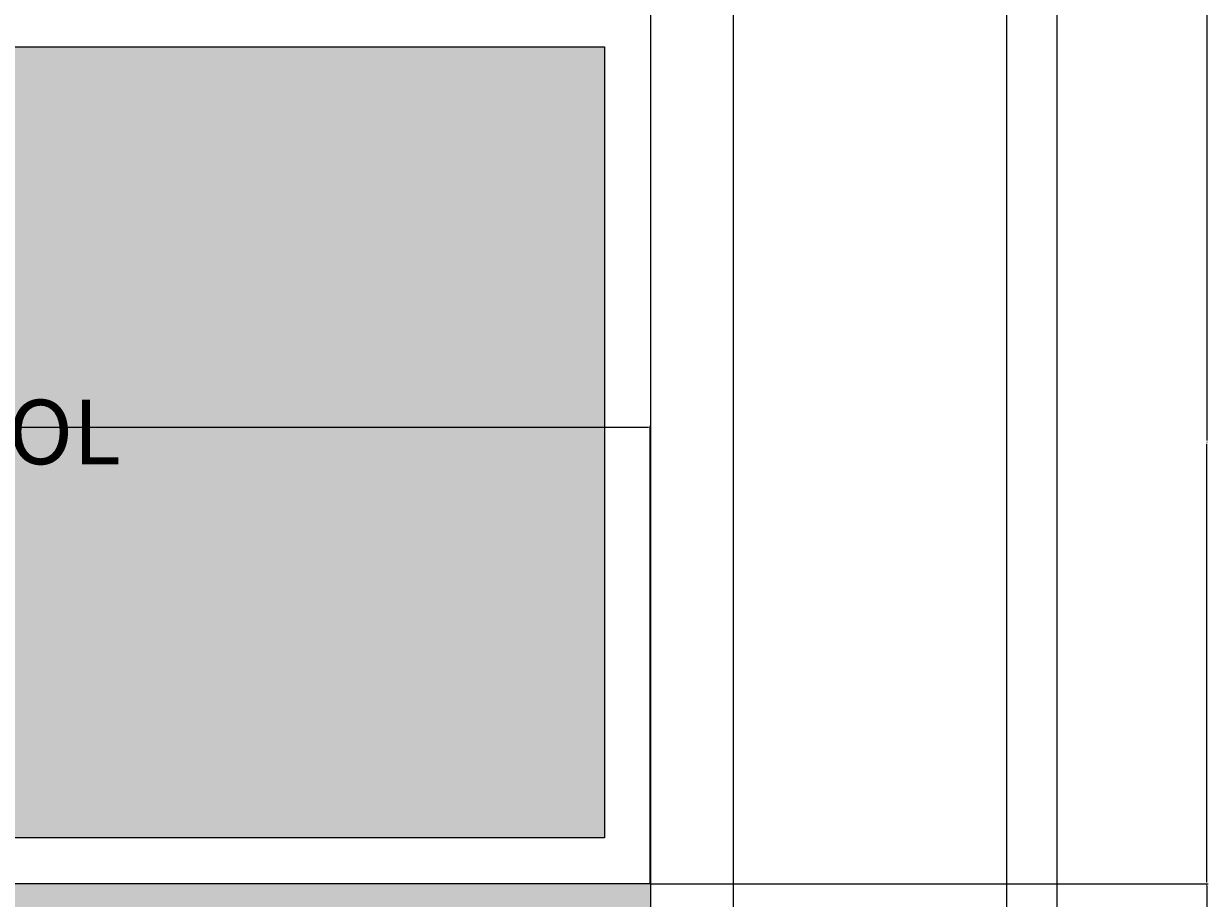
# Model space of a CAD drawing. Units: inches. Extents: x 84 to 1044, y -280 to 906.
# Tile 47 of 105: x 915 to 1044, y -66 to 29. Entities that reach past the tile are written whole.
import ezdxf

# ---------------------------------------------------------------- set-up
doc = ezdxf.new("R2010")
doc.units = ezdxf.units.IN
for name, color, linetype, lineweight in [('A-ANNO-DIMS', 2, 'Continuous', 18), ('A-ANNO-TTLB', 7, 'Continuous', 25), ('A-AREA-IDEN', 7, 'Continuous', 13), ('C-PROP', 7, 'Continuous', 25), ('L-POOL', 151, 'Continuous', 25), ('L-POOL-PATT', 143, 'Continuous', 9)]:
    doc.layers.add(name, color=color, linetype=linetype, lineweight=lineweight)
doc.layers.add('L-PLNT-PATT', color=9, linetype='Continuous', lineweight=9, true_color=0xafd9aa)
doc.styles.add('1-100DIM', font='txt', dxfattribs={"height": 0.3})
doc.styles.get("Standard").update_dxf_attribs({"font": 'arial.ttf'})
doc.dimstyles.get("Standard").update_dxf_attribs({"dimtxt": 0.18, "dimasz": 0.18, "dimexe": 0.18, "dimexo": 0.0625, "dimgap": 0.09, "dimtad": 0, "dimtih": 1, "dimtoh": 1, "dimdec": 4, "dimzin": 0, "dimdsep": 46, "dimtxsty": 'Standard', "dimcen": 0.09, "dimadec": 0, "dimazin": 0, "dimtfac": 1, "dimtdec": 4, "dimtofl": 0, "dimtmove": 0, "dimatfit": 3, "dimfxl": 1, "dimtolj": 1, "dimtzin": 0, "dimarcsym": 0})

# ---------------------------------------------------------------- blocks, each defined once
blk = doc.blocks.new('*D67')
at = {"layer": 'A-ANNO-DIMS', "color": 0, "lineweight": -2, "transparency": 16777216}
for p, q in [((791.07, -64.82), (791.07, -15.1)), ((791.25, -15.28), (886.79, -15.28)), ((982.89, -15.28), (887.35, -15.28)), ((983.07, -64.82), (983.07, -15.1))]:
    blk.add_line(p, q, dxfattribs=at)
at = {"layer": 'A-ANNO-DIMS', "color": 0, "transparency": 16777216}
for points in [[(791.25, -15.25), (791.25, -15.31), (791.07, -15.28)], [(982.89, -15.25), (982.89, -15.31), (983.07, -15.28)]]:
    blk.add_solid(points, dxfattribs=at)
at = {"layer": 'Defpoints', "color": 0, "transparency": 16777216}
for p in [(983.07, -15.28), (791.07, -64.88), (983.07, -64.88)]:
    blk.add_point(p, dxfattribs=at)
at = {"layer": 'A-ANNO-DIMS', "color": 0, "transparency": 16777216, "insert": (887.07, -15.28), "char_height": 0.18, "attachment_point": 5}
blk.add_mtext('\\A1;192', dxfattribs=at)
blk = doc.blocks.new('*D68')
at = {"layer": 'A-ANNO-DIMS', "color": 0, "lineweight": -2, "transparency": 16777216}
for p, q in [((983.14, 31.12), (1043.77, 31.12)), ((1043.59, 30.94), (1043.59, -16.7)), ((1043.59, -64.7), (1043.59, -17.06)), ((983.14, -64.88), (1043.77, -64.88))]:
    blk.add_line(p, q, dxfattribs=at)
at = {"layer": 'A-ANNO-DIMS', "color": 0, "transparency": 16777216}
for points in [[(1043.56, 30.94), (1043.62, 30.94), (1043.59, 31.12)], [(1043.56, -64.7), (1043.62, -64.7), (1043.59, -64.88)]]:
    blk.add_solid(points, dxfattribs=at)
at = {"layer": 'Defpoints', "color": 0, "transparency": 16777216}
for p in [(983.07, 31.12), (1043.59, 31.12), (983.07, -64.88)]:
    blk.add_point(p, dxfattribs=at)
at = {"layer": 'A-ANNO-DIMS', "color": 0, "transparency": 16777216, "insert": (1043.59, -16.88), "char_height": 0.18, "attachment_point": 5}
blk.add_mtext('\\A1;96', dxfattribs=at)
blk = doc.blocks.new('*D70')
at = {"layer": 'A-ANNO-DIMS', "color": 0, "lineweight": -2, "transparency": 16777216}
for p, q in [((983.14, -64.88), (1043.77, -64.88)), ((1043.59, -65.06), (1043.59, -93.2)), ((1043.59, -121.7), (1043.59, -93.56)), ((992.14, -121.88), (1043.77, -121.88))]:
    blk.add_line(p, q, dxfattribs=at)
at = {"layer": 'A-ANNO-DIMS', "color": 0, "transparency": 16777216}
for points in [[(1043.56, -65.06), (1043.62, -65.06), (1043.59, -64.88)], [(1043.56, -121.7), (1043.62, -121.7), (1043.59, -121.88)]]:
    blk.add_solid(points, dxfattribs=at)
at = {"layer": 'Defpoints', "color": 0, "transparency": 16777216}
for p in [(983.07, -64.88), (1043.59, -64.88), (992.07, -121.88)]:
    blk.add_point(p, dxfattribs=at)
at = {"layer": 'A-ANNO-DIMS', "color": 0, "transparency": 16777216, "insert": (1043.59, -93.38), "char_height": 0.18, "attachment_point": 5}
blk.add_mtext('\\A1;57', dxfattribs=at)

msp = doc.modelspace()

# ---------------------------------------------------------------- hatches: boundary and pattern name
at = {"layer": 'L-PLNT-PATT', "transparency": 33554597}
h = msp.add_hatch(color=256, dxfattribs=at)
h.dxf.hatch_style = 1
h.paths.add_polyline_path([(791.074, 31.12), (791.074, 91.12), (743.074, 91.12), (674.074, 91.12), (674.074, 31.12), (650.074, 31.12), (650.074, -112.88), (983.074, -112.88), (983.074, -64.88), (791.074, -64.88)])
at = {"layer": 'L-POOL-PATT', "transparency": 33554567}
h = msp.add_hatch(color=256, dxfattribs=at)
h.dxf.hatch_style = 1
h.set_gradient(color1=(122, 175, 223), color2=(39, 118, 187), name='INVCYLINDER')
h.paths.add_polyline_path([(978.074, 26.12), (796.074, 26.12), (796.074, -59.88), (978.074, -59.88)])

# ---------------------------------------------------------------- linework, layer by layer
at = {"layer": 'A-ANNO-TTLB'}
for points in [[(101.1, 905.916), (1027.308, 905.916), (1027.308, -279.764), (101.1, -279.764)], [(106.576, 900.439), (1021.832, 900.439), (1021.832, -274.288), (106.576, -274.288)]]:
    msp.add_lwpolyline(points, close=True, dxfattribs=at)
at = {"layer": 'C-PROP'}
for points in [[(143.179, -121.88), (134.179, -121.88), (134.179, 856.12), (992.074, 856.12), (992.074, -121.88), (624.574, -121.88)], [(143.179, -112.88), (143.179, 847.12), (983.074, 847.12), (983.074, -112.88), (624.574, -112.88)]]:
    msp.add_lwpolyline(points, dxfattribs=at)
at = {"layer": 'L-POOL'}
for points in [[(791.074, 31.12), (983.074, 31.12), (983.074, -64.88), (791.074, -64.88)], [(796.074, 26.12), (978.074, 26.12), (978.074, -59.88), (796.074, -59.88)]]:
    msp.add_lwpolyline(points, close=True, dxfattribs=at)

# ---------------------------------------------------------------- texts
at = {"layer": 'A-AREA-IDEN', "insert": (844.983, -12.265), "char_height": 7, "attachment_point": 1, "style": '1-100DIM'}
msp.add_mtext_dynamic_manual_height_columns('{\\f@Malgun Gothic|b0|i0|c0|p34;  SWIMMING POOL}', width=95.90564, gutter_width=15.851, heights=[0], dxfattribs=at)

# ---------------------------------------------------------------- dimensions: what is measured, and where the dimension line sits
at = {"layer": 'A-ANNO-DIMS'}
for base, p1, p2, angle, picture, middle in [((1043.588, 31.12), (983.074, -64.88), (983.074, 31.12), 90, '*D68', (1043.588, -16.88)), ((983.074, -15.28), (791.074, -64.88), (983.074, -64.88), 0, '*D67', (887.074, -15.28)), ((1043.588, -64.88), (992.074, -121.88), (983.074, -64.88), 90, '*D70', (1043.588, -93.38))]:
    dim = msp.add_linear_dim(base=base, p1=p1, p2=p2, angle=angle, dimstyle='Standard', override={"dimdec": 0, "dimlfac": 1, "dimrnd": 0, "dimzin": 0, "dimdsep": 46, "dimlunit": 2}, dxfattribs=at)
    dim.commit()
    dim.dimension.update_dxf_attribs({"geometry": picture, "text_midpoint": middle})

doc.saveas('drawing.dxf')
